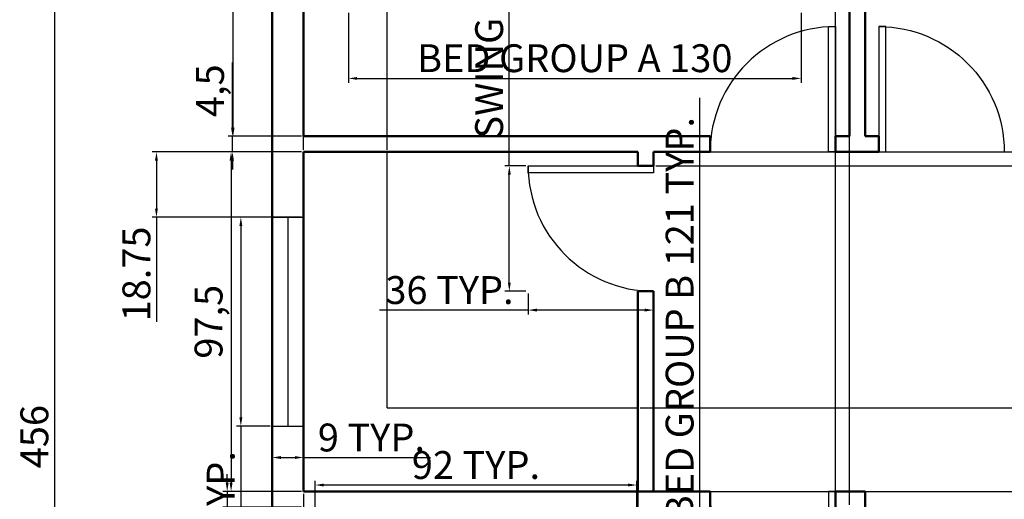
# Model space of a CAD drawing. Units: inches. Extents: x -349 to 9053, y 635 to 6001.
# Tile 3 of 7: x 257 to 540, y 880 to 1018. Entities that reach past the tile are written whole.
import ezdxf

# ---------------------------------------------------------------- set-up
doc = ezdxf.new("R2010")
doc.units = ezdxf.units.IN
for name, color, linetype, lineweight in [('A-ANNO-DIMS', 2, 'Continuous', 18), ('A-DOOR', 3, 'Continuous', 25), ('A-FLOR-CASE', 8, 'Continuous', 25), ('A-GLAZ', 4, 'Continuous', 25), ('A-WALL', 7, 'Continuous', 50)]:
    doc.layers.add(name, color=color, linetype=linetype, lineweight=lineweight)
doc.styles.get("Standard").update_dxf_attribs({"font": 'arial.ttf'})
doc.dimstyles.new('ISO-25', dxfattribs={"dimtxt": 8, "dimasz": 2.5, "dimexe": 1.25, "dimexo": 0.625, "dimtad": 1, "dimtxsty": 'Standard', "dimcen": 2.5, "dimadec": 0, "dimazin": 0, "dimtfac": 1, "dimtmove": 0, "dimatfit": 3, "dimfxl": 1, "dimarcsym": 0})

# ---------------------------------------------------------------- blocks, each defined once
blk = doc.blocks.new('*D9')
at = {"layer": 'A-ANNO-DIMS', "color": 0, "lineweight": -2, "transparency": 16777216}
for p, q in [((338.38, 1117), (317.52, 1117)), ((318.77, 986.75), (318.77, 1114.5)), ((338.38, 984.25), (317.52, 984.25))]:
    blk.add_line(p, q, dxfattribs=at)
at = {"layer": 'A-ANNO-DIMS', "color": 0, "transparency": 16777216}
for points in [[(318.36, 1114.5), (319.19, 1114.5), (318.77, 1117)], [(318.36, 986.75), (319.19, 986.75), (318.77, 984.25)]]:
    blk.add_solid(points, dxfattribs=at)
at = {"layer": 'Defpoints', "color": 0, "transparency": 16777216}
for p in [(318.77, 1117), (339, 1117), (339, 984.25)]:
    blk.add_point(p, dxfattribs=at)
at = {"layer": 'A-ANNO-DIMS', "color": 0, "transparency": 16777216, "insert": (313.34, 1050.62), "char_height": 8, "attachment_point": 5, "rotation": 90}
blk.add_mtext('132,75', dxfattribs=at)
blk = doc.blocks.new('*D10')
at = {"layer": 'A-ANNO-DIMS', "color": 0, "lineweight": -2, "transparency": 16777216}
for p, q in [((318.6, 986.75), (318.6, 1005.45)), ((338.38, 984.25), (317.35, 984.25)), ((318.6, 979.75), (318.6, 984.25)), ((338.38, 979.75), (317.35, 979.75)), ((318.6, 977.25), (318.6, 974.75))]:
    blk.add_line(p, q, dxfattribs=at)
at = {"layer": 'A-ANNO-DIMS', "color": 0, "transparency": 16777216}
for points in [[(318.18, 986.75), (319.02, 986.75), (318.6, 984.25)], [(318.18, 977.25), (319.02, 977.25), (318.6, 979.75)]]:
    blk.add_solid(points, dxfattribs=at)
at = {"layer": 'Defpoints', "color": 0, "transparency": 16777216}
for p in [(318.6, 984.25), (339, 984.25), (339, 979.75)]:
    blk.add_point(p, dxfattribs=at)
at = {"layer": 'A-ANNO-DIMS', "color": 0, "transparency": 16777216, "insert": (313.18, 997.35), "char_height": 8, "attachment_point": 5, "rotation": 90}
blk.add_mtext('4,5', dxfattribs=at)
blk = doc.blocks.new('*D11')
at = {"layer": 'A-ANNO-DIMS', "color": 0, "lineweight": -2, "transparency": 16777216}
for p, q in [((338.38, 979.75), (316.94, 979.75)), ((318.19, 977.25), (318.19, 884.75)), ((338.38, 882.25), (316.94, 882.25))]:
    blk.add_line(p, q, dxfattribs=at)
at = {"layer": 'A-ANNO-DIMS', "color": 0, "transparency": 16777216}
for points in [[(317.77, 977.25), (318.61, 977.25), (318.19, 979.75)], [(317.77, 884.75), (318.61, 884.75), (318.19, 882.25)]]:
    blk.add_solid(points, dxfattribs=at)
at = {"layer": 'Defpoints', "color": 0, "transparency": 16777216}
for p in [(339, 979.75), (318.19, 882.25), (339, 882.25)]:
    blk.add_point(p, dxfattribs=at)
at = {"layer": 'A-ANNO-DIMS', "color": 0, "transparency": 16777216, "insert": (312.76, 931), "char_height": 8, "attachment_point": 5, "rotation": 90}
blk.add_mtext('97,5', dxfattribs=at)
blk = doc.blocks.new('*D20')
at = {"layer": 'A-ANNO-DIMS', "color": 0, "lineweight": -2, "transparency": 16777216}
for p, q in [((317.08, 884.75), (317.08, 887.25)), ((338.38, 882.25), (315.83, 882.25)), ((317.08, 882.25), (317.08, 877.75)), ((338.38, 877.75), (315.83, 877.75)), ((317.08, 875.25), (317.08, 856.55))]:
    blk.add_line(p, q, dxfattribs=at)
at = {"layer": 'A-ANNO-DIMS', "color": 0, "transparency": 16777216}
for points in [[(316.66, 884.75), (317.5, 884.75), (317.08, 882.25)], [(316.66, 875.25), (317.5, 875.25), (317.08, 877.75)]]:
    blk.add_solid(points, dxfattribs=at)
at = {"layer": 'Defpoints', "color": 0, "transparency": 16777216}
for p in [(339, 882.25), (317.08, 877.75), (339, 877.75)]:
    blk.add_point(p, dxfattribs=at)
at = {"layer": 'A-ANNO-DIMS', "color": 0, "transparency": 16777216, "insert": (311.66, 864.65), "char_height": 8, "attachment_point": 5, "rotation": 90}
blk.add_mtext('4,5', dxfattribs=at)
blk = doc.blocks.new('*D31')
at = {"layer": 'A-ANNO-DIMS', "color": 0, "lineweight": -2, "transparency": 16777216}
for p, q in [((338.38, 1126), (266.19, 1126)), ((267.44, 1123.5), (267.44, 672.5)), ((338.38, 670), (266.19, 670))]:
    blk.add_line(p, q, dxfattribs=at)
at = {"layer": 'A-ANNO-DIMS', "color": 0, "transparency": 16777216}
for points in [[(267.02, 1123.5), (267.86, 1123.5), (267.44, 1126)], [(267.02, 672.5), (267.86, 672.5), (267.44, 670)]]:
    blk.add_solid(points, dxfattribs=at)
at = {"layer": 'Defpoints', "color": 0, "transparency": 16777216}
for p in [(339, 1126), (267.44, 670), (339, 670)]:
    blk.add_point(p, dxfattribs=at)
at = {"layer": 'A-ANNO-DIMS', "color": 0, "transparency": 16777216, "insert": (262.73, 898), "char_height": 8, "attachment_point": 5, "rotation": 90}
blk.add_mtext('456', dxfattribs=at)
blk = doc.blocks.new('DOOR-36IN-SWING')
blk.add_line((0, 0), (-2, 0))
blk.add_lwpolyline([(0, 36), (0, 0), (-2, 0), (-2, 36)], close=True)
blk.add_arc((0, 0), 36, 90, 180)
blk = doc.blocks.new('WIN-60IN')
for p, q in [((0, -4.5), (0, 4.5)), ((60, -4.5), (60, 4.5)), ((0, 0), (60, 0))]:
    blk.add_line(p, q)
blk = doc.blocks.new('*D43')
at = {"layer": 'A-ANNO-DIMS', "color": 0, "lineweight": -2, "transparency": 16777216}
for p, q in [((398.1, 975.75), (398.1, 1096.01)), ((402.88, 975.75), (396.85, 975.75)), ((398.1, 942.25), (398.1, 973.25)), ((402.88, 939.75), (396.85, 939.75))]:
    blk.add_line(p, q, dxfattribs=at)
at = {"layer": 'A-ANNO-DIMS', "color": 0, "transparency": 16777216}
for points in [[(397.68, 973.25), (398.52, 973.25), (398.1, 975.75)], [(397.68, 942.25), (398.52, 942.25), (398.1, 939.75)]]:
    blk.add_solid(points, dxfattribs=at)
at = {"layer": 'Defpoints', "color": 0, "transparency": 16777216}
for p in [(398.1, 975.75), (403.5, 975.75), (403.5, 939.75)]:
    blk.add_point(p, dxfattribs=at)
at = {"layer": 'A-ANNO-DIMS', "color": 0, "transparency": 16777216, "insert": (393.33, 1037.13), "char_height": 8, "attachment_point": 5, "rotation": 90}
blk.add_mtext('SWING DOOR 36 TYP.', dxfattribs=at)
blk = doc.blocks.new('*D44')
at = {"layer": 'A-ANNO-DIMS', "color": 0, "lineweight": -2, "transparency": 16777216}
for p, q in [((403.5, 939.12), (403.5, 933.1)), ((439.5, 939.12), (439.5, 933.1)), ((403.5, 934.35), (360.81, 934.35)), ((437, 934.35), (406, 934.35))]:
    blk.add_line(p, q, dxfattribs=at)
at = {"layer": 'A-ANNO-DIMS', "color": 0, "transparency": 16777216}
for points in [[(406, 934.77), (406, 933.93), (403.5, 934.35)], [(437, 934.77), (437, 933.93), (439.5, 934.35)]]:
    blk.add_solid(points, dxfattribs=at)
at = {"layer": 'Defpoints', "color": 0, "transparency": 16777216}
for p in [(403.5, 939.75), (439.5, 939.75), (403.5, 934.35)]:
    blk.add_point(p, dxfattribs=at)
at = {"layer": 'A-ANNO-DIMS', "color": 0, "transparency": 16777216, "insert": (380.91, 939.06), "char_height": 8, "attachment_point": 5}
blk.add_mtext('36 TYP.', dxfattribs=at)
blk = doc.blocks.new('*D45')
at = {"layer": 'A-ANNO-DIMS', "color": 0, "lineweight": -2, "transparency": 16777216}
for p, q in [((329.38, 961), (319.75, 961)), ((321, 958.5), (321, 903.5)), ((329.38, 901), (319.75, 901)), ((321, 901), (321, 785.97))]:
    blk.add_line(p, q, dxfattribs=at)
at = {"layer": 'A-ANNO-DIMS', "color": 0, "transparency": 16777216}
for points in [[(320.58, 958.5), (321.42, 958.5), (321, 961)], [(320.58, 903.5), (321.42, 903.5), (321, 901)]]:
    blk.add_solid(points, dxfattribs=at)
at = {"layer": 'Defpoints', "color": 0, "transparency": 16777216}
for p in [(330, 961), (321, 901), (330, 901)]:
    blk.add_point(p, dxfattribs=at)
at = {"layer": 'A-ANNO-DIMS', "color": 0, "transparency": 16777216, "insert": (316.24, 842.24), "char_height": 8, "attachment_point": 5, "rotation": 90}
blk.add_mtext('WINDOW W1 60 TYP.', dxfattribs=at)
blk = doc.blocks.new('*D46')
at = {"layer": 'A-ANNO-DIMS', "color": 0, "lineweight": -2, "transparency": 16777216}
for p, q in [((330, 900.38), (330, 890.75)), ((339, 900.38), (339, 890.75)), ((332.5, 892), (336.5, 892)), ((339, 892), (375.48, 892))]:
    blk.add_line(p, q, dxfattribs=at)
at = {"layer": 'A-ANNO-DIMS', "color": 0, "transparency": 16777216}
for points in [[(332.5, 892.42), (332.5, 891.58), (330, 892)], [(336.5, 892.42), (336.5, 891.58), (339, 892)]]:
    blk.add_solid(points, dxfattribs=at)
at = {"layer": 'Defpoints', "color": 0, "transparency": 16777216}
for p in [(330, 901), (339, 901), (339, 892)]:
    blk.add_point(p, dxfattribs=at)
at = {"layer": 'A-ANNO-DIMS', "color": 0, "transparency": 16777216, "insert": (358.49, 896.71), "char_height": 8, "attachment_point": 5}
blk.add_mtext('9 TYP.', dxfattribs=at)
blk = doc.blocks.new('*D49')
at = {"layer": 'A-ANNO-DIMS', "color": 0, "lineweight": -2, "transparency": 16777216}
for p, q in [((452.81, 865.99), (452.81, 995.27)), ((435.32, 865.99), (454.06, 865.99)), ((452.81, 747.7), (452.81, 863.49)), ((435.32, 745.2), (454.06, 745.2))]:
    blk.add_line(p, q, dxfattribs=at)
at = {"layer": 'A-ANNO-DIMS', "color": 0, "transparency": 16777216}
for points in [[(452.39, 863.49), (453.23, 863.49), (452.81, 865.99)], [(452.39, 747.7), (453.23, 747.7), (452.81, 745.2)]]:
    blk.add_solid(points, dxfattribs=at)
at = {"layer": 'Defpoints', "color": 0, "transparency": 16777216}
for p in [(434.69, 865.99), (452.81, 865.99), (434.69, 745.2)]:
    blk.add_point(p, dxfattribs=at)
at = {"layer": 'A-ANNO-DIMS', "color": 0, "transparency": 16777216, "insert": (448.04, 931.88), "char_height": 8, "attachment_point": 5, "rotation": 90}
blk.add_mtext('BED GROUP B 121 TYP.', dxfattribs=at)
blk = doc.blocks.new('*D50')
at = {"layer": 'A-ANNO-DIMS', "color": 0, "lineweight": -2, "transparency": 16777216}
for p, q in [((342.32, 866.61), (342.32, 885.35)), ((434.69, 866.61), (434.69, 885.35)), ((432.19, 884.1), (344.82, 884.1))]:
    blk.add_line(p, q, dxfattribs=at)
at = {"layer": 'A-ANNO-DIMS', "color": 0, "transparency": 16777216}
for points in [[(344.82, 884.52), (344.82, 883.69), (342.32, 884.1)], [(432.19, 884.52), (432.19, 883.69), (434.69, 884.1)]]:
    blk.add_solid(points, dxfattribs=at)
at = {"layer": 'Defpoints', "color": 0, "transparency": 16777216}
for p in [(342.32, 884.1), (342.32, 865.99), (434.69, 865.99)]:
    blk.add_point(p, dxfattribs=at)
at = {"layer": 'A-ANNO-DIMS', "color": 0, "transparency": 16777216, "insert": (388.51, 888.81), "char_height": 8, "attachment_point": 5}
blk.add_mtext('92 TYP.', dxfattribs=at)
blk = doc.blocks.new('*D53')
at = {"layer": 'A-ANNO-DIMS', "color": 0, "lineweight": -2, "transparency": 16777216}
for p, q in [((351.88, 1019.76), (351.88, 999.63)), ((481.9, 1019.76), (481.9, 999.63)), ((354.38, 1000.88), (479.4, 1000.88))]:
    blk.add_line(p, q, dxfattribs=at)
at = {"layer": 'A-ANNO-DIMS', "color": 0, "transparency": 16777216}
for points in [[(354.38, 1001.3), (354.38, 1000.47), (351.88, 1000.88)], [(479.4, 1001.3), (479.4, 1000.47), (481.9, 1000.88)]]:
    blk.add_solid(points, dxfattribs=at)
at = {"layer": 'Defpoints', "color": 0, "transparency": 16777216}
for p in [(351.88, 1020.39), (481.9, 1020.39), (481.9, 1000.88)]:
    blk.add_point(p, dxfattribs=at)
at = {"layer": 'A-ANNO-DIMS', "color": 0, "transparency": 16777216, "insert": (416.89, 1005.65), "char_height": 8, "attachment_point": 5}
blk.add_mtext('BED GROUP A 130', dxfattribs=at)
blk = doc.blocks.new('*D59')
at = {"layer": 'A-ANNO-DIMS', "color": 0, "lineweight": -2, "transparency": 16777216}
for p, q in [((435, 905.62), (435, 635.5)), ((339, 881.62), (339, 635.5)), ((341.5, 636.75), (432.5, 636.75))]:
    blk.add_line(p, q, dxfattribs=at)
at = {"layer": 'A-ANNO-DIMS', "color": 0, "transparency": 16777216}
for points in [[(341.5, 637.17), (341.5, 636.33), (339, 636.75)], [(432.5, 637.17), (432.5, 636.33), (435, 636.75)]]:
    blk.add_solid(points, dxfattribs=at)
at = {"layer": 'Defpoints', "color": 0, "transparency": 16777216}
for p in [(435, 906.25), (339, 882.25), (435, 636.75)]:
    blk.add_point(p, dxfattribs=at)
at = {"layer": 'A-ANNO-DIMS', "color": 0, "transparency": 16777216, "insert": (387, 641.46), "char_height": 8, "attachment_point": 5}
blk.add_mtext('96', dxfattribs=at)
blk = doc.blocks.new('*D60')
at = {"layer": 'A-ANNO-DIMS', "color": 0, "lineweight": -2, "transparency": 16777216}
for p, q in [((339, 980.38), (339, 1160.5)), ((363, 980.38), (363, 1160.5)), ((341.5, 1159.25), (360.5, 1159.25))]:
    blk.add_line(p, q, dxfattribs=at)
at = {"layer": 'A-ANNO-DIMS', "color": 0, "transparency": 16777216}
for points in [[(341.5, 1159.67), (341.5, 1158.83), (339, 1159.25)], [(360.5, 1159.67), (360.5, 1158.83), (363, 1159.25)]]:
    blk.add_solid(points, dxfattribs=at)
at = {"layer": 'Defpoints', "color": 0, "transparency": 16777216}
for p in [(363, 1159.25), (339, 979.75), (363, 979.75)]:
    blk.add_point(p, dxfattribs=at)
at = {"layer": 'A-ANNO-DIMS', "color": 0, "transparency": 16777216, "insert": (351, 1163.89), "char_height": 8, "attachment_point": 5}
blk.add_mtext('24', dxfattribs=at)
blk = doc.blocks.new('*D61')
at = {"layer": 'A-ANNO-DIMS', "color": 0, "lineweight": -2, "transparency": 16777216}
for p, q in [((435.63, 906.25), (748.6, 906.25)), ((747.35, 884.75), (747.35, 903.75)), ((435.63, 882.25), (748.6, 882.25))]:
    blk.add_line(p, q, dxfattribs=at)
at = {"layer": 'A-ANNO-DIMS', "color": 0, "transparency": 16777216}
for points in [[(746.93, 903.75), (747.76, 903.75), (747.35, 906.25)], [(746.93, 884.75), (747.76, 884.75), (747.35, 882.25)]]:
    blk.add_solid(points, dxfattribs=at)
at = {"layer": 'Defpoints', "color": 0, "transparency": 16777216}
for p in [(435, 906.25), (747.35, 906.25), (435, 882.25)]:
    blk.add_point(p, dxfattribs=at)
at = {"layer": 'A-ANNO-DIMS', "color": 0, "transparency": 16777216, "insert": (742.71, 894.25), "char_height": 8, "attachment_point": 5, "rotation": 90}
blk.add_mtext('24', dxfattribs=at)
blk = doc.blocks.new('*D62')
at = {"layer": 'A-ANNO-DIMS', "color": 0, "lineweight": -2, "transparency": 16777216}
for p, q in [((338.38, 979.75), (295.5, 979.75)), ((296.75, 977.25), (296.75, 963.5)), ((338.38, 961), (295.5, 961)), ((296.75, 961), (296.75, 930.95))]:
    blk.add_line(p, q, dxfattribs=at)
at = {"layer": 'A-ANNO-DIMS', "color": 0, "transparency": 16777216}
for points in [[(296.33, 977.25), (297.17, 977.25), (296.75, 979.75)], [(296.33, 963.5), (297.17, 963.5), (296.75, 961)]]:
    blk.add_solid(points, dxfattribs=at)
at = {"layer": 'Defpoints', "color": 0, "transparency": 16777216}
for p in [(339, 979.75), (296.75, 961), (339, 961)]:
    blk.add_point(p, dxfattribs=at)
at = {"layer": 'A-ANNO-DIMS', "color": 0, "transparency": 16777216, "insert": (292.04, 944.72), "char_height": 8, "attachment_point": 5, "rotation": 90}
blk.add_mtext('18.75', dxfattribs=at)
blk = doc.blocks.new('*D63')
at = {"layer": 'A-ANNO-DIMS', "color": 0, "lineweight": -2, "transparency": 16777216}
for p, q in [((747.35, 982.25), (747.35, 984.75)), ((440.13, 979.75), (748.6, 979.75)), ((747.35, 979.75), (747.35, 975.75)), ((440.13, 975.75), (748.6, 975.75)), ((747.35, 973.25), (747.35, 963.97))]:
    blk.add_line(p, q, dxfattribs=at)
at = {"layer": 'A-ANNO-DIMS', "color": 0, "transparency": 16777216}
for points in [[(746.93, 982.25), (747.76, 982.25), (747.35, 979.75)], [(746.93, 973.25), (747.76, 973.25), (747.35, 975.75)]]:
    blk.add_solid(points, dxfattribs=at)
at = {"layer": 'Defpoints', "color": 0, "transparency": 16777216}
for p in [(439.5, 979.75), (439.5, 975.75), (747.35, 975.75)]:
    blk.add_point(p, dxfattribs=at)
at = {"layer": 'A-ANNO-DIMS', "color": 0, "transparency": 16777216, "insert": (742.72, 967.36), "char_height": 8, "attachment_point": 5, "rotation": 90}
blk.add_mtext('4', dxfattribs=at)
blk = doc.blocks.new('*D76')
at = {"layer": 'A-ANNO-DIMS', "color": 0, "lineweight": -2, "transparency": 16777216}
for p, q in [((491.75, 878.37), (491.75, 1160.5)), ((495.75, 878.37), (495.75, 1160.5)), ((489.25, 1159.25), (479.97, 1159.25)), ((495.75, 1159.25), (491.75, 1159.25)), ((498.25, 1159.25), (500.75, 1159.25))]:
    blk.add_line(p, q, dxfattribs=at)
at = {"layer": 'A-ANNO-DIMS', "color": 0, "transparency": 16777216}
for points in [[(489.25, 1159.67), (489.25, 1158.83), (491.75, 1159.25)], [(498.25, 1159.67), (498.25, 1158.83), (495.75, 1159.25)]]:
    blk.add_solid(points, dxfattribs=at)
at = {"layer": 'Defpoints', "color": 0, "transparency": 16777216}
for p in [(491.75, 1159.25), (491.75, 877.75), (495.75, 877.75)]:
    blk.add_point(p, dxfattribs=at)
at = {"layer": 'A-ANNO-DIMS', "color": 0, "transparency": 16777216, "insert": (483.36, 1163.88), "char_height": 8, "attachment_point": 5}
blk.add_mtext('4', dxfattribs=at)

msp = doc.modelspace()

# ---------------------------------------------------------------- linework, layer by layer
at = {"layer": 'A-FLOR-CASE'}
for p, q in [((363, 906.25), (363, 979.75)), ((363, 906.25), (435, 906.25)), ((339, 882.25), (435, 882.25))]:
    msp.add_line(p, q, dxfattribs=at)
at = {"layer": 'A-WALL'}
for p, q in [((330, 1126), (330, 670)), ((339, 1117), (339, 984.25)), ((339, 1117), (339, 984.25)), ((495.75, 1117), (495.75, 984.25)), ((500.25, 1117), (500.25, 984.25)), ((339, 984.25), (455.75, 984.25)), ((455.75, 984.25), (455.75, 979.75)), ((491.75, 984.25), (491.75, 979.75)), ((491.75, 984.25), (495.75, 984.25)), ((500.25, 984.25), (504.25, 984.25)), ((504.25, 984.25), (504.25, 979.75)), ((339, 979.75), (435, 979.75)), ((339, 882.25), (339, 979.75)), ((339, 979.75), (339, 882.25)), ((339, 979.75), (339, 882.25)), ((435, 975.75), (435, 979.75)), ((439.5, 975.75), (439.5, 979.75)), ((439.5, 979.75), (455.75, 979.75)), ((491.75, 979.75), (498, 979.75)), ((498, 979.75), (504.25, 979.75)), ((435, 975.75), (439.5, 975.75)), ((435, 882.25), (435, 939.75)), ((435, 939.75), (439.5, 939.75)), ((439.5, 882.25), (439.5, 939.75)), ((339, 882.25), (455.75, 882.25)), ((455.75, 877.75), (455.75, 882.25)), ((491.75, 877.75), (491.75, 882.25)), ((491.75, 882.25), (495.75, 882.25)), ((495.75, 882.25), (500.25, 882.25)), ((500.25, 882.25), (500.25, 798.25))]:
    msp.add_line(p, q, dxfattribs=at)

# ---------------------------------------------------------------- block references
at = {"layer": 'A-DOOR'}
msp.add_blockref('DOOR-36IN-SWING', (491.75, 979.75), dxfattribs=at)
at = {"layer": 'A-DOOR', "extrusion": (0, 0, -1), "zscale": -1}
msp.add_blockref('DOOR-36IN-SWING', (-504.25, 979.75), dxfattribs=at)
at = {"layer": 'A-DOOR', "rotation": 89.99999999999952}
msp.add_blockref('DOOR-36IN-SWING', (439.5, 975.75), dxfattribs=at)
at = {"layer": 'A-DOOR', "extrusion": (0, 0, -1), "zscale": -1, "rotation": 180}
msp.add_blockref('DOOR-36IN-SWING', (-491.75, 882.25), dxfattribs=at)
at = {"layer": 'A-GLAZ', "rotation": 270.0000000000001}
msp.add_blockref('WIN-60IN', (334.5, 961), dxfattribs=at)

# ---------------------------------------------------------------- dimensions: what is measured, and where the dimension line sits
at = {"layer": 'A-ANNO-DIMS'}
for base, p1, p2, picture, middle in [((363, 1159.25), (339, 979.75), (363, 979.75), '*D60', (351, 1163.8914)), ((491.75, 1159.25), (495.75, 877.75), (491.75, 877.75), '*D76', (483.3583, 1163.875)), ((435, 636.75), (339, 882.25), (435, 906.25), '*D59', (387, 641.4596))]:
    dim = msp.add_linear_dim(base=base, p1=p1, p2=p2, dimstyle='ISO-25', override={"dimdec": 0, "dimlfac": 1, "dimrnd": 0, "dimzin": 0, "dimdsep": 46, "dimlunit": 2}, dxfattribs=at)
    dim.commit()
    dim.dimension.update_dxf_attribs({"geometry": picture, "text_midpoint": middle})
for base, p1, p2, override, picture, middle in [((267.4414, 670), (339, 1126), (339, 670), {"dimclrd": 0, "dimclre": 0, "dimclrt": 0}, '*D31', (262.7318, 898)), ((318.7745, 1117), (339, 984.25), (339, 1117), {"dimclrd": 0, "dimclre": 0, "dimclrt": 0}, '*D9', (313.3419, 1050.625)), ((318.5986, 984.25), (339, 979.75), (339, 984.25), {"dimclrd": 0, "dimclre": 0, "dimclrt": 0}, '*D10', (313.1824, 997.3484)), ((747.3471, 975.75), (439.5, 979.75), (439.5, 975.75), {"dimdec": 0, "dimlfac": 1, "dimrnd": 0, "dimzin": 0, "dimdsep": 46, "dimlunit": 2}, '*D63', (742.7221, 967.3583)), ((296.75, 961), (339, 979.75), (339, 961), {"dimdec": 2, "dimlfac": 1, "dimrnd": 0, "dimzin": 0, "dimdsep": 46, "dimlunit": 2}, '*D62', (292.0404, 944.7236)), ((318.1907, 882.25), (339, 979.75), (339, 882.25), {"dimclrd": 0, "dimclre": 0, "dimclrt": 0}, '*D11', (312.7581, 931)), ((747.3471, 906.25), (435, 882.25), (435, 906.25), {"dimdec": 0, "dimlfac": 1, "dimrnd": 0, "dimzin": 0, "dimdsep": 46, "dimlunit": 2}, '*D61', (742.7057, 894.25)), ((317.0807, 877.75), (339, 882.25), (339, 877.75), {"dimclrd": 0, "dimclre": 0, "dimclrt": 0}, '*D20', (311.6645, 864.6516))]:
    dim = msp.add_linear_dim(base=base, p1=p1, p2=p2, angle=90, dimstyle='ISO-25', override=override, dxfattribs=at)
    dim.commit()
    dim.dimension.update_dxf_attribs({"geometry": picture, "text_midpoint": middle})
for base, p1, p2, angle, text, picture, middle in [((398.1, 975.75), (403.5, 939.75), (403.5, 975.75), 90, 'SWING DOOR <> TYP.', '*D43', (393.3331, 1037.1315)), ((452.8083, 865.9867), (434.6907, 745.2023), (434.6907, 865.9867), 90, 'BED GROUP B <> TYP.', '*D49', (448.0442, 931.8784)), ((321, 901), (330, 961), (330, 901), 270, 'WINDOW W1 <> TYP.', '*D45', (316.2358, 842.2352)), ((403.5, 934.35), (439.5, 939.75), (403.5, 939.75), 180, '<> TYP.', '*D44', (380.9071, 939.0623)), ((342.3245, 884.1043), (434.6907, 865.9867), (342.3245, 865.9867), 180, '<> TYP.', '*D50', (388.5076, 888.8139))]:
    dim = msp.add_linear_dim(base=base, p1=p1, p2=p2, angle=angle, text=text, dimstyle='ISO-25', override={"dimdec": 0, "dimlfac": 1, "dimrnd": 0, "dimzin": 0, "dimdsep": 46, "dimlunit": 2}, dxfattribs=at)
    dim.commit()
    dim.dimension.update_dxf_attribs({"geometry": picture, "text_midpoint": middle})
for base, p1, p2, text, picture, middle in [((481.8989, 1000.8847), (351.8813, 1020.3874), (481.8989, 1020.3874), 'BED GROUP A <>', '*D53', (416.8901, 1005.6516)), ((339, 892), (330, 901), (339, 901), '<> TYP.', '*D46', (358.4879, 896.7096))]:
    dim = msp.add_linear_dim(base=base, p1=p1, p2=p2, text=text, dimstyle='ISO-25', override={"dimdec": 0, "dimlfac": 1, "dimrnd": 0, "dimzin": 0, "dimdsep": 46, "dimlunit": 2}, dxfattribs=at)
    dim.commit()
    dim.dimension.update_dxf_attribs({"geometry": picture, "text_midpoint": middle})

doc.saveas('drawing.dxf')
